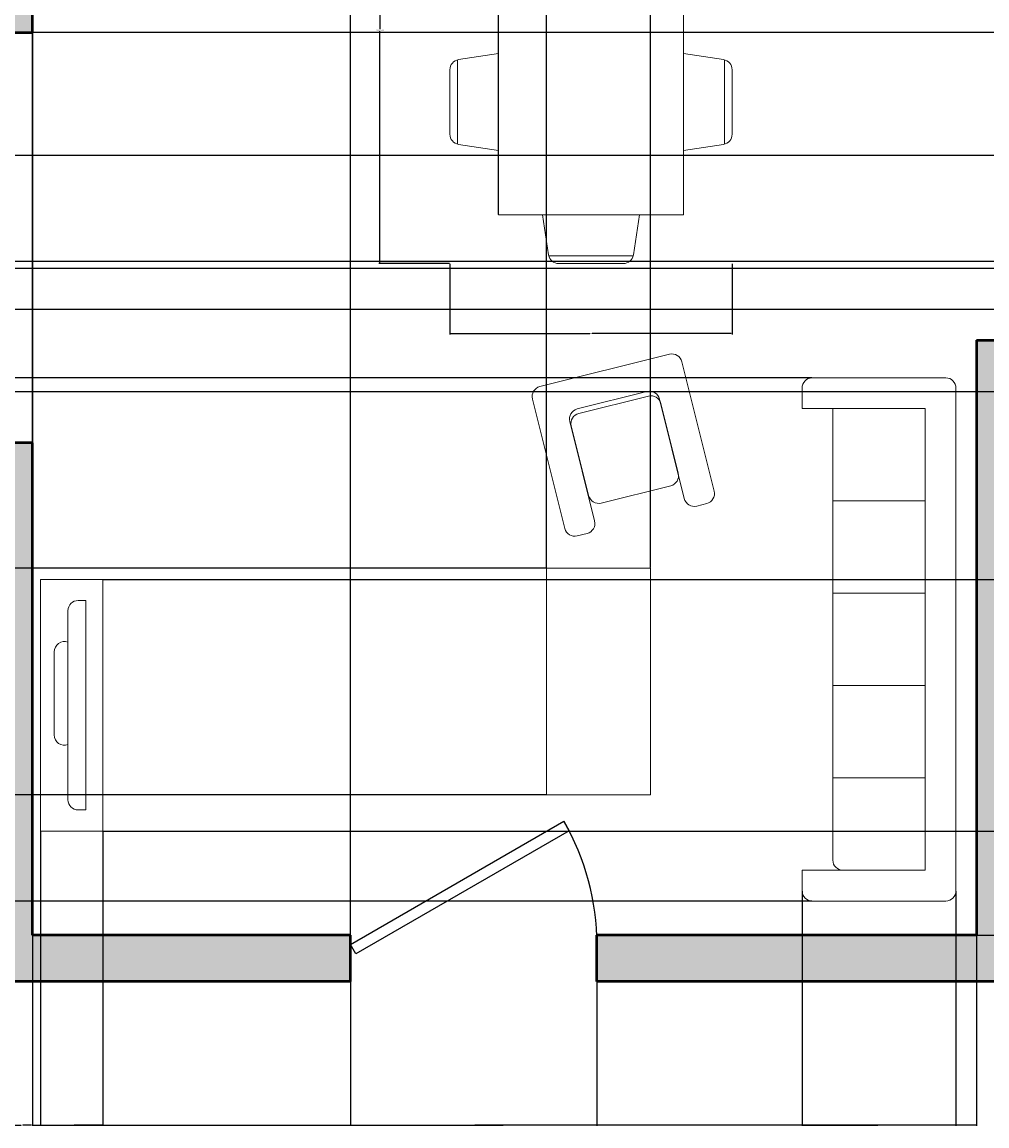
# Model space of a CAD drawing. Units: inches. Extents: x 1869 to 2483, y 2084 to 2479.
# Tile 5 of 7: x 2088 to 2276, y 2084 to 2299. Entities that reach past the tile are written whole.
import ezdxf

# ---------------------------------------------------------------- set-up
doc = ezdxf.new("R2010")
doc.units = ezdxf.units.IN
for name, color, linetype, lineweight in [('A-ANNO-DIMS', 2, 'Continuous', 18), ('A-DOOR', 3, 'Continuous', 25), ('A-EQPM', 8, 'Continuous', 18), ('A-FURN', 8, 'Continuous', 18), ('A-WALL', 7, 'Continuous', 50)]:
    doc.layers.add(name, color=color, linetype=linetype, lineweight=lineweight)
doc.layers.add('A-WALL-PATT', color=18, linetype='Continuous', lineweight=13, true_color=0x000000)
doc.styles.get("Standard").update_dxf_attribs({"font": 'arial.ttf'})
doc.dimstyles.get("Standard").update_dxf_attribs({"dimtxt": 0.18, "dimasz": 0.18, "dimexe": 0.18, "dimexo": 0.0625, "dimgap": 0.09, "dimtad": 0, "dimtih": 1, "dimtoh": 1, "dimdec": 4, "dimzin": 0, "dimdsep": 46, "dimtxsty": 'Standard', "dimcen": 0.09, "dimadec": 0, "dimazin": 0, "dimtfac": 1, "dimtdec": 4, "dimtofl": 0, "dimtmove": 0, "dimatfit": 3, "dimfxl": 1, "dimtolj": 1, "dimtzin": 0, "dimarcsym": 0})

# ---------------------------------------------------------------- blocks, each defined once
blk = doc.blocks.new('Dining Set - 36 x 72 in.')
for p, q in [((-22.23, 26), (-5.76, 26)), ((-20.29, 27.5), (-7.71, 27.5)), ((5.77, 26), (22.24, 26)), ((7.71, 27.5), (20.29, 27.5)), ((-22.26, 25.81), (-23.48, 18)), ((-4.52, 18), (-5.74, 25.81)), ((5.74, 25.81), (4.52, 18)), ((23.48, 18), (22.26, 25.81)), ((36, 18), (-36, 18)), ((-36, 18), (-36, -18)), ((36, -18), (36, 18)), ((-43.81, 8.26), (-36, 9.48)), ((43.81, 8.26), (36, 9.48)), ((-44, 8.23), (-44, -8.24)), ((44, 8.23), (44, -8.24)), ((-45.5, 6.29), (-45.5, -6.29)), ((45.5, 6.29), (45.5, -6.29)), ((-36, -9.48), (-43.81, -8.26)), ((36, -9.48), (43.81, -8.26)), ((-36, -18), (36, -18)), ((-22.26, -25.81), (-23.48, -18)), ((-4.52, -18), (-5.74, -25.81)), ((5.74, -25.81), (4.52, -18)), ((23.48, -18), (22.26, -25.81)), ((-22.23, -26), (-5.76, -26)), ((-20.29, -27.5), (-7.71, -27.5)), ((5.77, -26), (22.24, -26)), ((7.71, -27.5), (20.29, -27.5))]:
    blk.add_line(p, q)
for centre, start, end in [((-20.29, 25.5), 90, 171.1198), ((-7.71, 25.5), 8.881, 90), ((7.71, 25.5), 90, 171.1198), ((20.29, 25.5), 8.881, 90), ((-43.5, 6.29), 98.8806, 180), ((43.5, 6.29), 0, 81.1194), ((-43.5, -6.29), 180, 261.1194), ((43.5, -6.29), 278.8806, 0), ((-20.29, -25.5), 188.8802, 270), ((-7.71, -25.5), 270, 351.1191), ((7.71, -25.5), 188.8802, 270), ((20.29, -25.5), 270, 351.1191)]:
    blk.add_arc(centre, 2, start, end)
blk = doc.blocks.new('*U10')
for p, q in [((0, 0), (0, -6)), ((40, 0), (40, -6))]:
    blk.add_line(p, q)
blk.add_lwpolyline([(0, 0), (34.64, 20), (35.52, 18.48), (0.87, -1.52)], close=True)
blk.add_arc((0, 0), 40, 0, 30)
blk = doc.blocks.new('*D29')
at = {"layer": 'A-ANNO-DIMS', "color": 0, "lineweight": -2, "transparency": 16777216}
for p, q in [((2171.37, 2342.65), (2157.61, 2342.65)), ((2157.79, 2342.47), (2157.79, 2297.33)), ((2157.79, 2251.83), (2157.79, 2296.97)), ((2171.37, 2251.65), (2157.61, 2251.65))]:
    blk.add_line(p, q, dxfattribs=at)
at = {"layer": 'A-ANNO-DIMS', "color": 0, "transparency": 16777216}
for points in [[(2157.76, 2342.47), (2157.82, 2342.47), (2157.79, 2342.65)], [(2157.76, 2251.83), (2157.82, 2251.83), (2157.79, 2251.65)]]:
    blk.add_solid(points, dxfattribs=at)
at = {"layer": 'Defpoints', "color": 0, "transparency": 16777216}
for p in [(2171.44, 2342.65), (2157.79, 2251.65), (2171.44, 2251.65)]:
    blk.add_point(p, dxfattribs=at)
at = {"layer": 'A-ANNO-DIMS', "color": 0, "transparency": 16777216, "insert": (2157.79, 2297.15), "char_height": 0.18, "attachment_point": 5}
blk.add_mtext('\\A1;DINING SET 91', dxfattribs=at)
blk = doc.blocks.new('*D30')
at = {"layer": 'A-ANNO-DIMS', "color": 0, "lineweight": -2, "transparency": 16777216}
for p, q in [((2171.44, 2251.59), (2171.44, 2237.82)), ((2226.44, 2251.59), (2226.44, 2237.82)), ((2171.62, 2238), (2198.72, 2238)), ((2226.26, 2238), (2199.16, 2238))]:
    blk.add_line(p, q, dxfattribs=at)
at = {"layer": 'A-ANNO-DIMS', "color": 0, "transparency": 16777216}
for points in [[(2171.62, 2238.03), (2171.62, 2237.97), (2171.44, 2238)], [(2226.26, 2238.03), (2226.26, 2237.97), (2226.44, 2238)]]:
    blk.add_solid(points, dxfattribs=at)
at = {"layer": 'Defpoints', "color": 0, "transparency": 16777216}
for p in [(2171.44, 2251.65), (2226.44, 2251.65), (2226.44, 2238)]:
    blk.add_point(p, dxfattribs=at)
at = {"layer": 'A-ANNO-DIMS', "color": 0, "transparency": 16777216, "insert": (2198.94, 2238), "char_height": 0.18, "attachment_point": 5}
blk.add_mtext('\\A1;55', dxfattribs=at)
blk = doc.blocks.new('*D41')
at = {"layer": 'A-ANNO-DIMS', "color": 0, "lineweight": -2, "transparency": 16777216}
for p, q in [((2090.08, 2120.66), (2090.08, 2083.54)), ((2274.08, 2120.66), (2274.08, 2083.54)), ((2090.26, 2083.72), (2181.8, 2083.72)), ((2273.9, 2083.72), (2182.36, 2083.72))]:
    blk.add_line(p, q, dxfattribs=at)
at = {"layer": 'A-ANNO-DIMS', "color": 0, "transparency": 16777216}
for points in [[(2090.26, 2083.75), (2090.26, 2083.69), (2090.08, 2083.72)], [(2273.9, 2083.75), (2273.9, 2083.69), (2274.08, 2083.72)]]:
    blk.add_solid(points, dxfattribs=at)
at = {"layer": 'Defpoints', "color": 0, "transparency": 16777216}
for p in [(2090.08, 2120.72), (2274.08, 2120.72), (2274.08, 2083.72)]:
    blk.add_point(p, dxfattribs=at)
at = {"layer": 'A-ANNO-DIMS', "color": 0, "transparency": 16777216, "insert": (2182.08, 2083.72), "char_height": 0.18, "attachment_point": 5}
blk.add_mtext('\\A1;184', dxfattribs=at)
blk = doc.blocks.new('*D54')
at = {"layer": 'A-ANNO-DIMS', "color": 0, "lineweight": -2, "transparency": 16777216}
for p, q in [((2152.08, 2111.66), (2152.08, 2083.54)), ((2200.08, 2111.66), (2200.08, 2083.54)), ((2152.26, 2083.72), (2175.86, 2083.72)), ((2199.9, 2083.72), (2176.3, 2083.72))]:
    blk.add_line(p, q, dxfattribs=at)
at = {"layer": 'A-ANNO-DIMS', "color": 0, "transparency": 16777216}
for points in [[(2152.26, 2083.75), (2152.26, 2083.69), (2152.08, 2083.72)], [(2199.9, 2083.75), (2199.9, 2083.69), (2200.08, 2083.72)]]:
    blk.add_solid(points, dxfattribs=at)
at = {"layer": 'Defpoints', "color": 0, "transparency": 16777216}
for p in [(2152.08, 2111.72), (2200.08, 2111.72), (2200.08, 2083.72)]:
    blk.add_point(p, dxfattribs=at)
at = {"layer": 'A-ANNO-DIMS', "color": 0, "transparency": 16777216, "insert": (2176.08, 2083.72), "char_height": 0.18, "attachment_point": 5}
blk.add_mtext('\\A1;48', dxfattribs=at)
blk = doc.blocks.new('*D55')
at = {"layer": 'A-ANNO-DIMS', "color": 0, "lineweight": -2, "transparency": 16777216}
for p, q in [((2090.08, 2120.79), (2090.08, 2479.07)), ((2090.26, 2478.89), (2120.86, 2478.89)), ((2151.9, 2478.89), (2121.3, 2478.89)), ((2152.08, 2120.79), (2152.08, 2479.07))]:
    blk.add_line(p, q, dxfattribs=at)
at = {"layer": 'A-ANNO-DIMS', "color": 0, "transparency": 16777216}
for points in [[(2090.26, 2478.92), (2090.26, 2478.86), (2090.08, 2478.89)], [(2151.9, 2478.92), (2151.9, 2478.86), (2152.08, 2478.89)]]:
    blk.add_solid(points, dxfattribs=at)
at = {"layer": 'Defpoints', "color": 0, "transparency": 16777216}
for p in [(2152.08, 2478.89), (2090.08, 2120.72), (2152.08, 2120.72)]:
    blk.add_point(p, dxfattribs=at)
at = {"layer": 'A-ANNO-DIMS', "color": 0, "transparency": 16777216, "insert": (2121.08, 2478.89), "char_height": 0.18, "attachment_point": 5}
blk.add_mtext('\\A1;62', dxfattribs=at)
blk = doc.blocks.new('*D57')
at = {"layer": 'A-ANNO-DIMS', "color": 0, "lineweight": -2, "transparency": 16777216}
for p, q in [((2446.02, 2296.72), (1868.9, 2296.72)), ((1869.08, 2296.54), (1869.08, 2274.58)), ((1869.08, 2252.25), (1869.08, 2274.22)), ((2446.02, 2252.07), (1868.9, 2252.07))]:
    blk.add_line(p, q, dxfattribs=at)
at = {"layer": 'A-ANNO-DIMS', "color": 0, "transparency": 16777216}
for points in [[(1869.05, 2296.54), (1869.11, 2296.54), (1869.08, 2296.72)], [(1869.05, 2252.25), (1869.11, 2252.25), (1869.08, 2252.07)]]:
    blk.add_solid(points, dxfattribs=at)
at = {"layer": 'Defpoints', "color": 0, "transparency": 16777216}
for p in [(1869.08, 2296.72), (2446.08, 2296.72), (2446.08, 2252.07)]:
    blk.add_point(p, dxfattribs=at)
at = {"layer": 'A-ANNO-DIMS', "color": 0, "transparency": 16777216, "insert": (1869.08, 2274.4), "char_height": 0.18, "attachment_point": 5}
blk.add_mtext('\\A1;44.65', dxfattribs=at)
blk = doc.blocks.new('*D63')
at = {"layer": 'A-ANNO-DIMS', "color": 0, "lineweight": -2, "transparency": 16777216}
for p, q in [((2348.34, 2272.72), (1868.9, 2272.72)), ((1869.08, 2272.54), (1869.08, 2257.91)), ((1869.08, 2242.9), (1869.08, 2257.54)), ((2348.34, 2242.72), (1868.9, 2242.72))]:
    blk.add_line(p, q, dxfattribs=at)
at = {"layer": 'A-ANNO-DIMS', "color": 0, "transparency": 16777216}
for points in [[(1869.05, 2272.54), (1869.11, 2272.54), (1869.08, 2272.72)], [(1869.05, 2242.9), (1869.11, 2242.9), (1869.08, 2242.72)]]:
    blk.add_solid(points, dxfattribs=at)
at = {"layer": 'Defpoints', "color": 0, "transparency": 16777216}
for p in [(1869.08, 2272.72), (2348.4, 2272.72), (2348.4, 2242.72)]:
    blk.add_point(p, dxfattribs=at)
at = {"layer": 'A-ANNO-DIMS', "color": 0, "transparency": 16777216, "insert": (1869.08, 2257.72), "char_height": 0.18, "attachment_point": 5}
blk.add_mtext('\\A1;30', dxfattribs=at)
blk = doc.blocks.new('*D68')
at = {"layer": 'A-ANNO-DIMS', "color": 0, "lineweight": -2, "transparency": 16777216}
for p, q in [((2010.14, 2250.72), (2483.26, 2250.72)), ((2483.08, 2250.54), (2483.08, 2238.9)), ((2483.08, 2226.9), (2483.08, 2238.54)), ((2010.14, 2226.72), (2483.26, 2226.72))]:
    blk.add_line(p, q, dxfattribs=at)
at = {"layer": 'A-ANNO-DIMS', "color": 0, "transparency": 16777216}
for points in [[(2483.05, 2250.54), (2483.11, 2250.54), (2483.08, 2250.72)], [(2483.05, 2226.9), (2483.11, 2226.9), (2483.08, 2226.72)]]:
    blk.add_solid(points, dxfattribs=at)
at = {"layer": 'Defpoints', "color": 0, "transparency": 16777216}
for p in [(2010.08, 2250.72), (2483.08, 2250.72), (2010.08, 2226.72)]:
    blk.add_point(p, dxfattribs=at)
at = {"layer": 'A-ANNO-DIMS', "color": 0, "transparency": 16777216, "insert": (2483.08, 2238.72), "char_height": 0.18, "attachment_point": 5}
blk.add_mtext('\\A1;24', dxfattribs=at)
blk = doc.blocks.new('*D72')
at = {"layer": 'A-ANNO-DIMS', "color": 0, "lineweight": -2, "transparency": 16777216}
for p, q in [((2086.08, 2300.66), (2086.08, 2083.54)), ((2090.08, 2296.66), (2090.08, 2083.54)), ((2086.26, 2083.72), (2087.93, 2083.72)), ((2089.9, 2083.72), (2088.23, 2083.72))]:
    blk.add_line(p, q, dxfattribs=at)
at = {"layer": 'A-ANNO-DIMS', "color": 0, "transparency": 16777216}
for points in [[(2086.26, 2083.75), (2086.26, 2083.69), (2086.08, 2083.72)], [(2089.9, 2083.75), (2089.9, 2083.69), (2090.08, 2083.72)]]:
    blk.add_solid(points, dxfattribs=at)
at = {"layer": 'Defpoints', "color": 0, "transparency": 16777216}
for p in [(2086.08, 2300.72), (2090.08, 2296.72), (2090.08, 2083.72)]:
    blk.add_point(p, dxfattribs=at)
at = {"layer": 'A-ANNO-DIMS', "color": 0, "transparency": 16777216, "insert": (2088.08, 2083.72), "char_height": 0.18, "attachment_point": 5}
blk.add_mtext('\\A1;4', dxfattribs=at)
blk = doc.blocks.new('*D73')
at = {"layer": 'A-ANNO-DIMS', "color": 0, "lineweight": -2, "transparency": 16777216}
for p, q in [((2200.14, 2120.72), (2483.26, 2120.72)), ((2483.08, 2120.54), (2483.08, 2116.41)), ((2483.08, 2111.9), (2483.08, 2116.04)), ((2200.14, 2111.72), (2483.26, 2111.72))]:
    blk.add_line(p, q, dxfattribs=at)
at = {"layer": 'A-ANNO-DIMS', "color": 0, "transparency": 16777216}
for points in [[(2483.05, 2120.54), (2483.11, 2120.54), (2483.08, 2120.72)], [(2483.05, 2111.9), (2483.11, 2111.9), (2483.08, 2111.72)]]:
    blk.add_solid(points, dxfattribs=at)
at = {"layer": 'Defpoints', "color": 0, "transparency": 16777216}
for p in [(2200.08, 2120.72), (2483.08, 2120.72), (2200.08, 2111.72)]:
    blk.add_point(p, dxfattribs=at)
at = {"layer": 'A-ANNO-DIMS', "color": 0, "transparency": 16777216, "insert": (2483.08, 2116.22), "char_height": 0.18, "attachment_point": 5}
blk.add_mtext('\\A1;9', dxfattribs=at)
blk = doc.blocks.new('*D86')
at = {"layer": 'A-ANNO-DIMS', "color": 0, "lineweight": -2, "transparency": 16777216}
for p, q in [((2241.99, 2229.37), (1868.9, 2229.37)), ((1869.08, 2229.19), (1869.08, 2178.55)), ((1869.08, 2127.55), (1869.08, 2178.19)), ((2241.99, 2127.37), (1868.9, 2127.37))]:
    blk.add_line(p, q, dxfattribs=at)
at = {"layer": 'A-ANNO-DIMS', "color": 0, "transparency": 16777216}
for points in [[(1869.05, 2229.19), (1869.11, 2229.19), (1869.08, 2229.37)], [(1869.05, 2127.55), (1869.11, 2127.55), (1869.08, 2127.37)]]:
    blk.add_solid(points, dxfattribs=at)
at = {"layer": 'Defpoints', "color": 0, "transparency": 16777216}
for p in [(2242.05, 2229.37), (1869.08, 2127.37), (2242.05, 2127.37)]:
    blk.add_point(p, dxfattribs=at)
at = {"layer": 'A-ANNO-DIMS', "color": 0, "transparency": 16777216, "insert": (1869.08, 2178.37), "char_height": 0.18, "attachment_point": 5}
blk.add_mtext('\\A1;102', dxfattribs=at)
blk = doc.blocks.new('*D87')
at = {"layer": 'A-ANNO-DIMS', "color": 0, "lineweight": -2, "transparency": 16777216}
for p, q in [((2240.05, 2129.31), (2240.05, 2083.54)), ((2270.05, 2129.31), (2270.05, 2083.54)), ((2240.23, 2083.72), (2254.84, 2083.72)), ((2269.87, 2083.72), (2255.27, 2083.72))]:
    blk.add_line(p, q, dxfattribs=at)
at = {"layer": 'A-ANNO-DIMS', "color": 0, "transparency": 16777216}
for points in [[(2240.23, 2083.75), (2240.23, 2083.69), (2240.05, 2083.72)], [(2269.87, 2083.75), (2269.87, 2083.69), (2270.05, 2083.72)]]:
    blk.add_solid(points, dxfattribs=at)
at = {"layer": 'Defpoints', "color": 0, "transparency": 16777216}
for p in [(2240.05, 2129.37), (2270.05, 2129.37), (2270.05, 2083.72)]:
    blk.add_point(p, dxfattribs=at)
at = {"layer": 'A-ANNO-DIMS', "color": 0, "transparency": 16777216, "insert": (2255.05, 2083.72), "char_height": 0.18, "attachment_point": 5}
blk.add_mtext('\\A1;30', dxfattribs=at)
blk = doc.blocks.new('*D90')
at = {"layer": 'A-ANNO-DIMS', "color": 0, "lineweight": -2, "transparency": 16777216}
for p, q in [((2190.22, 2192.3), (1868.9, 2192.3)), ((1869.08, 2192.12), (1869.08, 2170.36)), ((1869.08, 2148.24), (1869.08, 2170)), ((2190.22, 2148.06), (1868.9, 2148.06))]:
    blk.add_line(p, q, dxfattribs=at)
at = {"layer": 'A-ANNO-DIMS', "color": 0, "transparency": 16777216}
for points in [[(1869.05, 2192.12), (1869.11, 2192.12), (1869.08, 2192.3)], [(1869.05, 2148.24), (1869.11, 2148.24), (1869.08, 2148.06)]]:
    blk.add_solid(points, dxfattribs=at)
at = {"layer": 'Defpoints', "color": 0, "transparency": 16777216}
for p in [(1869.08, 2192.3), (2190.29, 2192.3), (2190.29, 2148.06)]:
    blk.add_point(p, dxfattribs=at)
at = {"layer": 'A-ANNO-DIMS', "color": 0, "transparency": 16777216, "insert": (1869.08, 2170.18), "char_height": 0.18, "attachment_point": 5}
blk.add_mtext('\\A1;44.24', dxfattribs=at)
blk = doc.blocks.new('*D91')
at = {"layer": 'A-ANNO-DIMS', "color": 0, "lineweight": -2, "transparency": 16777216}
for p, q in [((2190.29, 2192.37), (2190.29, 2479.07)), ((2190.47, 2478.89), (2199.94, 2478.89)), ((2210.34, 2478.89), (2200.87, 2478.89)), ((2210.52, 2192.37), (2210.52, 2479.07))]:
    blk.add_line(p, q, dxfattribs=at)
at = {"layer": 'A-ANNO-DIMS', "color": 0, "transparency": 16777216}
for points in [[(2190.47, 2478.92), (2190.47, 2478.86), (2190.29, 2478.89)], [(2210.34, 2478.92), (2210.34, 2478.86), (2210.52, 2478.89)]]:
    blk.add_solid(points, dxfattribs=at)
at = {"layer": 'Defpoints', "color": 0, "transparency": 16777216}
for p in [(2210.52, 2478.89), (2190.29, 2192.3), (2210.52, 2192.3)]:
    blk.add_point(p, dxfattribs=at)
at = {"layer": 'A-ANNO-DIMS', "color": 0, "transparency": 16777216, "insert": (2200.4, 2478.89), "char_height": 0.18, "attachment_point": 5}
blk.add_mtext('\\A1;20.236', dxfattribs=at)
blk = doc.blocks.new('*D92')
at = {"layer": 'A-ANNO-DIMS', "color": 0, "lineweight": -2, "transparency": 16777216}
for p, q in [((2091.7, 2140.95), (2091.7, 2083.54)), ((2103.84, 2140.95), (2103.84, 2083.54)), ((2091.88, 2083.72), (2097.31, 2083.72)), ((2103.66, 2083.72), (2098.22, 2083.72))]:
    blk.add_line(p, q, dxfattribs=at)
at = {"layer": 'A-ANNO-DIMS', "color": 0, "transparency": 16777216}
for points in [[(2091.88, 2083.75), (2091.88, 2083.69), (2091.7, 2083.72)], [(2103.66, 2083.75), (2103.66, 2083.69), (2103.84, 2083.72)]]:
    blk.add_solid(points, dxfattribs=at)
at = {"layer": 'Defpoints', "color": 0, "transparency": 16777216}
for p in [(2091.7, 2141.01), (2103.84, 2141.01), (2103.84, 2083.72)]:
    blk.add_point(p, dxfattribs=at)
at = {"layer": 'A-ANNO-DIMS', "color": 0, "transparency": 16777216, "insert": (2097.77, 2083.72), "char_height": 0.18, "attachment_point": 5}
blk.add_mtext('\\A1;12.142', dxfattribs=at)
blk = doc.blocks.new('*D93')
at = {"layer": 'A-ANNO-DIMS', "color": 0, "lineweight": -2, "transparency": 16777216}
for p, q in [((2103.9, 2190.06), (2483.26, 2190.06)), ((2483.08, 2189.88), (2483.08, 2165.72)), ((2483.08, 2141.19), (2483.08, 2165.36)), ((2103.9, 2141.01), (2483.26, 2141.01))]:
    blk.add_line(p, q, dxfattribs=at)
at = {"layer": 'A-ANNO-DIMS', "color": 0, "transparency": 16777216}
for points in [[(2483.05, 2189.88), (2483.11, 2189.88), (2483.08, 2190.06)], [(2483.05, 2141.19), (2483.11, 2141.19), (2483.08, 2141.01)]]:
    blk.add_solid(points, dxfattribs=at)
at = {"layer": 'Defpoints', "color": 0, "transparency": 16777216}
for p in [(2103.84, 2190.06), (2483.08, 2190.06), (2103.84, 2141.01)]:
    blk.add_point(p, dxfattribs=at)
at = {"layer": 'A-ANNO-DIMS', "color": 0, "transparency": 16777216, "insert": (2483.08, 2165.54), "char_height": 0.18, "attachment_point": 5}
blk.add_mtext('\\A1;49.05', dxfattribs=at)
blk = doc.blocks.new('*D95')
at = {"layer": 'A-ANNO-DIMS', "color": 0, "lineweight": -2, "transparency": 16777216}
for p, q in [((2090.08, 2296.79), (2090.08, 2479.07)), ((2090.26, 2478.89), (2135.11, 2478.89)), ((2180.76, 2478.89), (2135.9, 2478.89)), ((2180.94, 2261.21), (2180.94, 2479.07))]:
    blk.add_line(p, q, dxfattribs=at)
at = {"layer": 'A-ANNO-DIMS', "color": 0, "transparency": 16777216}
for points in [[(2090.26, 2478.92), (2090.26, 2478.86), (2090.08, 2478.89)], [(2180.76, 2478.92), (2180.76, 2478.86), (2180.94, 2478.89)]]:
    blk.add_solid(points, dxfattribs=at)
at = {"layer": 'Defpoints', "color": 0, "transparency": 16777216}
for p in [(2180.94, 2478.89), (2090.08, 2296.72), (2180.94, 2261.15)]:
    blk.add_point(p, dxfattribs=at)
at = {"layer": 'A-ANNO-DIMS', "color": 0, "transparency": 16777216, "insert": (2135.51, 2478.89), "char_height": 0.18, "attachment_point": 5}
blk.add_mtext('\\A1;90.86', dxfattribs=at)

msp = doc.modelspace()

# ---------------------------------------------------------------- hatches: boundary and pattern name
at = {"layer": 'A-WALL-PATT'}
h = msp.add_hatch(color=256, dxfattribs=at)
h.dxf.hatch_style = 1
h.paths.add_polyline_path([(2373.5248, 2429.7235), (2046.5221, 2429.7235), (2046.5221, 2420.7235), (2086.0799, 2420.7235), (2086.0799, 2330.7235), (2086.0799, 2300.7235), (2080.0799, 2300.7235), (2080.0799, 2296.7235), (2090.0799, 2296.7235), (2090.0799, 2374.7235), (2170.0799, 2374.7235), (2170.0799, 2378.7235), (2090.0799, 2378.7235), (2090.0799, 2420.7235), (2322.0799, 2420.7235), (2322.0799, 2378.7235), (2242.0799, 2378.7235), (2242.0799, 2374.7235), (2322.0799, 2374.7235), (2322.0799, 2336.7235), (2326.0799, 2336.7235), (2326.0799, 2420.7235), (2373.5248, 2420.7235)])
h = msp.add_hatch(color=256, dxfattribs=at)
h.dxf.hatch_style = 1
h.paths.add_polyline_path([(2342.287, 2120.7235), (2278.0799, 2120.7235), (2278.0799, 2192.7235), (2278.0799, 2232.7235), (2284.0799, 2232.7235), (2284.0799, 2236.7235), (2274.0799, 2236.7235), (2274.0799, 2120.7235), (2200.0799, 2120.7235), (2200.0799, 2111.7235), (2342.287, 2111.7235)])
h = msp.add_hatch(color=256, dxfattribs=at)
h.dxf.hatch_style = 1
h.paths.add_polyline_path([(2152.0799, 2118.9235), (2152.0799, 2120.7235), (2090.0799, 2120.7235), (2090.0799, 2216.7235), (2080.1689, 2216.7235), (2080.1689, 2212.7235), (2086.0799, 2212.7235), (2086.0799, 2120.7235), (2010.3331, 2120.7235), (2010.3331, 2111.7235), (2152.0799, 2111.7235)])

# ---------------------------------------------------------------- linework, layer by layer
at = {"layer": 'A-EQPM'}
msp.add_lwpolyline([(2100.4783, 2185.9743), (2099.0151, 2185.9743, 0.41421356), (2097.0151, 2183.9743), (2097.0151, 2147.1297, 0.41421356), (2099.0151, 2145.1297), (2100.4783, 2145.1297)], format="xyb", close=True, dxfattribs=at)
msp.add_lwpolyline([(2097.0151, 2151.8547), (2097.0151, 2182.3151)], dxfattribs=at)
msp.add_lwpolyline([(2097.0151, 2177.8515, 0.51847329), (2094.3435, 2175.9677), (2094.3435, 2159.7533, 0.51847329), (2097.0151, 2157.8695)], format="xyb", dxfattribs=at)
at = {"layer": 'A-FURN'}
for p, q in [((2214.212, 2233.962), (2188.9855, 2227.6673)), ((2216.6367, 2232.5057), (2222.9314, 2207.2792)), ((2242.0537, 2229.3727), (2268.0537, 2229.3727)), ((2240.0537, 2227.3727), (2240.0537, 2223.3727)), ((2270.0537, 2227.3727), (2270.0537, 2133.3727)), ((2187.5292, 2225.2426), (2193.8239, 2200.0161)), ((2209.8431, 2226.6879), (2196.2596, 2223.2984)), ((2212.2678, 2225.2316), (2217.1099, 2205.8266)), ((2240.0537, 2223.3727), (2264.0537, 2223.3727)), ((2264.0537, 2223.3727), (2264.0537, 2133.3727)), ((2194.8033, 2220.8737), (2199.6454, 2201.4687)), ((2219.5347, 2204.3703), (2221.4752, 2204.8545)), ((2196.2487, 2198.5598), (2198.1892, 2199.044)), ((2264.0537, 2133.3727), (2240.0537, 2133.3727)), ((2240.0537, 2133.3727), (2240.0537, 2129.3727)), ((2270.0537, 2133.3727), (2270.0537, 2129.3727)), ((2268.0537, 2127.3727), (2242.0537, 2127.3727))]:
    msp.add_line(p, q, dxfattribs=at)
msp.add_lwpolyline([(2196.5437, 2222.4149), (2210.1272, 2225.8044, -0.41421356), (2212.5519, 2224.3481), (2215.9414, 2210.7646, -0.41421356), (2214.4851, 2208.3399), (2200.9016, 2204.9504, -0.41421356), (2198.4769, 2206.4067), (2195.0875, 2219.9902, -0.41421356)], format="xyb", close=True, dxfattribs=at)
msp.add_lwpolyline([(2264.0537, 2223.3727), (2246.0537, 2223.3727), (2246.0537, 2135.3727, 0.41421356), (2248.0537, 2133.3727), (2264.0537, 2133.3727), (2264.0537, 2151.3727)], format="xyb", dxfattribs=at)
for points in [[(2264.0537, 2205.3727), (2246.0537, 2205.3727), (2246.0537, 2187.3727), (2264.0537, 2187.3727)], [(2190.2869, 2192.3029), (2210.5231, 2192.3029), (2210.5231, 2148.0595), (2190.2869, 2148.0595)], [(2103.8391, 2190.0613), (2091.6973, 2190.0613), (2091.6973, 2141.0143), (2103.8391, 2141.0143)], [(2264.0537, 2187.3727), (2246.0537, 2187.3727), (2246.0537, 2169.3727), (2264.0537, 2169.3727)], [(2264.0537, 2169.3727), (2246.0537, 2169.3727), (2246.0537, 2151.3727), (2264.0537, 2151.3727)]]:
    msp.add_lwpolyline(points, close=True, dxfattribs=at)
for centre, start, end in [((2214.6962, 2232.0215), 14.010839, 104.010839), ((2242.0537, 2227.3727), 90, 180), ((2268.0537, 2227.3727), 0, 90), ((2189.4697, 2225.7268), 104.010839, 194.010839), ((2210.3273, 2224.7474), 14.010839, 104.010839), ((2196.7438, 2221.3579), 104.010839, 194.010839), ((2219.0504, 2206.3108), 194.010839, 284.010839), ((2220.9909, 2206.795), 284.010839, 14.010839), ((2197.7049, 2200.9845), 284.010839, 14.010839), ((2195.7644, 2200.5003), 194.010839, 284.010839), ((2242.0537, 2129.3727), 180, 270), ((2268.0537, 2129.3727), 270, 0)]:
    msp.add_arc(centre, 2, start, end, dxfattribs=at)
at = {"layer": 'A-WALL'}
for p, q in [((2090.0799, 2296.7235), (2090.0799, 2374.7235)), ((2080.0799, 2296.7235), (2090.0799, 2296.7235)), ((2274.0799, 2236.7235), (2274.0799, 2120.7235)), ((2274.0799, 2236.7235), (2284.0799, 2236.7235)), ((2090.0799, 2216.7235), (2080.1689, 2216.7235)), ((2090.0799, 2120.7235), (2090.0799, 2216.7235)), ((2152.0799, 2120.7235), (2090.0799, 2120.7235)), ((2152.0799, 2111.7235), (2152.0799, 2120.7235)), ((2274.0799, 2120.7235), (2200.0799, 2120.7235)), ((2200.0799, 2111.7235), (2200.0799, 2120.7235))]:
    msp.add_line(p, q, dxfattribs=at)
msp.add_lwpolyline([(2152.0799, 2111.7235), (1897.0799, 2111.7235), (1897.0799, 2429.7235), (2455.0799, 2429.7235), (2455.0799, 2111.7235), (2200.0799, 2111.7235)], dxfattribs=at)

# ---------------------------------------------------------------- block references
at = {"layer": 'A-DOOR', "xscale": 1.199999999999999, "yscale": 1.199999999999999, "zscale": 1.199999999999999}
msp.add_blockref('*U10', (2152.0799, 2118.9235), dxfattribs=at)
at = {"layer": 'A-FURN', "rotation": 270}
msp.add_blockref('Dining Set - 36 x 72 in.', (2198.9372, 2297.1488), dxfattribs=at)

# ---------------------------------------------------------------- dimensions: what is measured, and where the dimension line sits
at = {"layer": 'A-ANNO-DIMS'}
for base, p1, p2, override, picture, middle in [((2152.0799, 2478.8871), (2090.0799, 2120.7235), (2152.0799, 2120.7235), {"dimdec": 0, "dimlfac": 1, "dimrnd": 0, "dimzin": 0, "dimdsep": 46, "dimlunit": 2}, '*D55', (2121.0799, 2478.8871)), ((2180.9372, 2478.8871), (2090.0799, 2296.7235), (2180.9372, 2261.1488), {"dimdec": 2, "dimlfac": 1, "dimrnd": 0, "dimzin": 0, "dimdsep": 46, "dimlunit": 2}, '*D95', (2135.5085, 2478.8871)), ((2210.5231, 2478.8871), (2190.2869, 2192.3029), (2210.5231, 2192.3029), {"dimdec": 3, "dimlfac": 1, "dimrnd": 0, "dimzin": 0, "dimdsep": 46, "dimlunit": 2}, '*D91', (2200.405, 2478.8871)), ((2090.0799, 2083.7235), (2086.0799, 2300.7235), (2090.0799, 2296.7235), {"dimdec": 0, "dimlfac": 1, "dimrnd": 0, "dimzin": 0, "dimdsep": 46, "dimlunit": 2}, '*D72', (2088.0799, 2083.7235)), ((2226.4372, 2237.9988), (2171.4372, 2251.6488), (2226.4372, 2251.6488), {"dimdec": 0, "dimlfac": 1, "dimrnd": 0, "dimzin": 0, "dimdsep": 46, "dimlunit": 2}, '*D30', (2198.9372, 2237.9988)), ((2103.8391, 2083.7235), (2091.6973, 2141.0143), (2103.8391, 2141.0143), {"dimdec": 3, "dimlfac": 1, "dimrnd": 0, "dimzin": 0, "dimdsep": 46, "dimlunit": 2}, '*D92', (2097.7682, 2083.7235)), ((2270.0537, 2083.7235), (2240.0537, 2129.3727), (2270.0537, 2129.3727), {"dimdec": 0, "dimlfac": 1, "dimrnd": 0, "dimzin": 0, "dimdsep": 46, "dimlunit": 2}, '*D87', (2255.0537, 2083.7235)), ((2274.0799, 2083.7235), (2090.0799, 2120.7235), (2274.0799, 2120.7235), {"dimdec": 0, "dimlfac": 1, "dimrnd": 0, "dimzin": 0, "dimdsep": 46, "dimlunit": 2}, '*D41', (2182.0799, 2083.7235)), ((2200.0799, 2083.7235), (2152.0799, 2111.7235), (2200.0799, 2111.7235), {"dimdec": 0, "dimlfac": 1, "dimrnd": 0, "dimzin": 0, "dimdsep": 46, "dimlunit": 2}, '*D54', (2176.0799, 2083.7235))]:
    dim = msp.add_linear_dim(base=base, p1=p1, p2=p2, dimstyle='Standard', override=override, dxfattribs=at)
    dim.commit()
    dim.dimension.update_dxf_attribs({"geometry": picture, "text_midpoint": middle})
dim = msp.add_linear_dim(base=(2157.7872, 2251.6488), p1=(2171.4372, 2342.6488), p2=(2171.4372, 2251.6488), angle=270, text='DINING SET <>', dimstyle='Standard', override={"dimdec": 0, "dimlfac": 1, "dimrnd": 0, "dimzin": 0, "dimdsep": 46, "dimlunit": 2}, dxfattribs=at)
dim.commit()
dim.dimension.update_dxf_attribs({"geometry": '*D29', "text_midpoint": (2157.7872, 2297.1488)})
for base, p1, p2, override, picture, middle in [((1869.0799, 2296.7235), (2446.0799, 2252.0706), (2446.0799, 2296.7235), {"dimdec": 2, "dimlfac": 1, "dimrnd": 0, "dimzin": 0, "dimdsep": 46, "dimlunit": 2}, '*D57', (1869.0799, 2274.3971)), ((1869.0799, 2272.7235), (2348.3982, 2242.7235), (2348.3982, 2272.7235), {"dimdec": 0, "dimlfac": 1, "dimrnd": 0, "dimzin": 0, "dimdsep": 46, "dimlunit": 2}, '*D63', (1869.0799, 2257.7235)), ((2483.0799, 2250.7235), (2010.0799, 2226.7235), (2010.0799, 2250.7235), {"dimdec": 0, "dimlfac": 1, "dimrnd": 0, "dimzin": 0, "dimdsep": 46, "dimlunit": 2}, '*D68', (2483.0799, 2238.7235)), ((1869.0799, 2127.3727), (2242.0537, 2229.3727), (2242.0537, 2127.3727), {"dimdec": 0, "dimlfac": 1, "dimrnd": 0, "dimzin": 0, "dimdsep": 46, "dimlunit": 2}, '*D86', (1869.0799, 2178.3727)), ((1869.0799, 2192.3029), (2190.2869, 2148.0595), (2190.2869, 2192.3029), {"dimdec": 2, "dimlfac": 1, "dimrnd": 0, "dimzin": 0, "dimdsep": 46, "dimlunit": 2}, '*D90', (1869.0799, 2170.1812)), ((2483.0799, 2190.0613), (2103.8391, 2141.0143), (2103.8391, 2190.0613), {"dimdec": 2, "dimlfac": 1, "dimrnd": 0, "dimzin": 0, "dimdsep": 46, "dimlunit": 2}, '*D93', (2483.0799, 2165.5378)), ((2483.0799, 2120.7235), (2200.0799, 2111.7235), (2200.0799, 2120.7235), {"dimdec": 0, "dimlfac": 1, "dimrnd": 0, "dimzin": 0, "dimdsep": 46, "dimlunit": 2}, '*D73', (2483.0799, 2116.2235))]:
    dim = msp.add_linear_dim(base=base, p1=p1, p2=p2, angle=90, dimstyle='Standard', override=override, dxfattribs=at)
    dim.commit()
    dim.dimension.update_dxf_attribs({"geometry": picture, "text_midpoint": middle})

doc.saveas('drawing.dxf')
